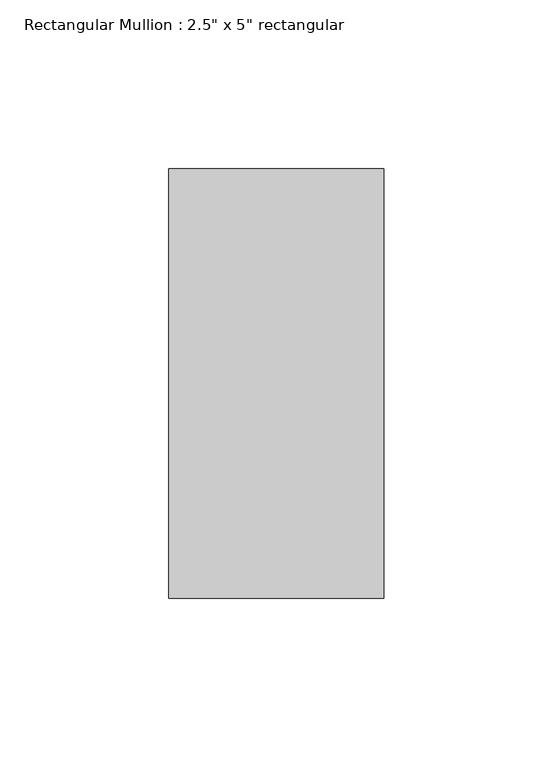
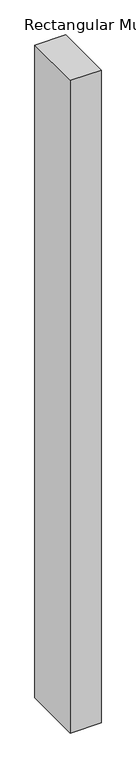
"""IFC4 building model written with IfcOpenShell, lengths in millimetres: member geometry."""

from ifc_helpers import new_model, si_unit, frame, origin, place, context, project, spatial, polyline, outline, extrude, source, transform, mapped, element, save


def member_26d67f61(model_context):
    return source(origin(), model_context, "Body", "SweptSolid", [
        extrude(outline(polyline([(0.0, 63.5), (0.0, -63.5), (-63.5, -63.5), (-63.5, 63.5), (0.0, 63.5)])), frame((0.0, 0.0, -1428.75), z_axis=(0.0, 0.0, 1.0), x_axis=(1.0, 0.0, 0.0)), (0.0, 0.0, 1.0), 1428.75),
    ])


if __name__ == "__main__":
    model = new_model("IFC4")
    model_context = context("Model", 3, world=origin())
    ifc_project = project(units=[si_unit("LENGTHUNIT", "METRE", prefix="MILLI")], contexts=[model_context])
    site = spatial("IfcSite", under=ifc_project)
    building = spatial("IfcBuilding", under=site)
    placement = place(None, origin())
    member_shape = member_26d67f61(model_context)
    element("IfcMember", 1, ObjectType="Rectangular Mullion : 2.5\" x 5\" rectangular", at=placement, inside=building, context=model_context, shape_type="MappedRepresentation", body=[
        mapped(member_shape, transform((0.0, 0.0, 0.0), x_axis=(1.0, 0.0, 0.0), y_axis=(0.0, 1.0, 0.0), z_axis=(0.0, 0.0, 1.0))),
    ])
    save(model, "model.ifc")

# Revit data of these elements
# Type "Rectangular Mullion : 2.5\" x 5\" rectangular"
#   built-in parameter 1007304 = 0.416667 (stored number, unit not read)
#   built-in parameter 1007301 = 0.104167 (stored number, unit not read)
#   built-in parameter 1007300 = 0.104167 (stored number, unit not read)
# Element 1 (IfcMember, "Rectangular Mullion : 2.5\" x 5\" rectangular")
#   Materials on its faces: "Aluminum"
# Materials
#   "Aluminum": class "Metal", colour RGB 247 247 247, transparency 0, Description = "Aluminum 6061", Cost = 0
